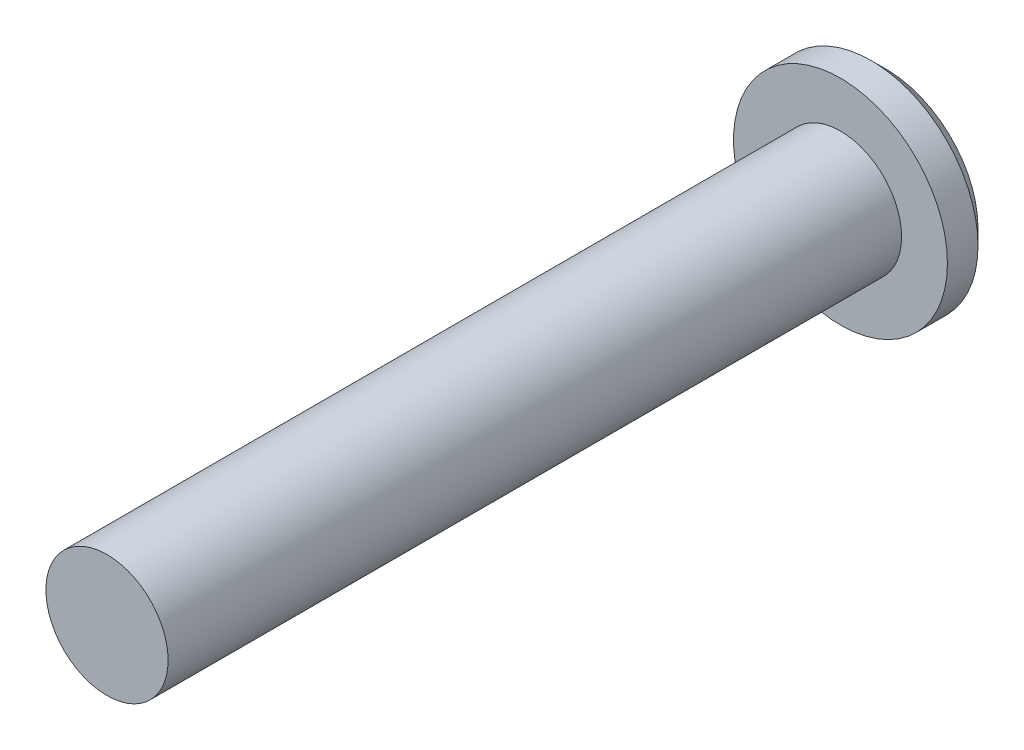
ISO-10303-21;
HEADER;
FILE_DESCRIPTION(('STEP AP214'),'2;1');
FILE_NAME('part.step','',(''),(''),'','','');
FILE_SCHEMA(('AUTOMOTIVE_DESIGN { 1 0 10303 214 1 1 1 1 }'));
ENDSEC;
DATA;
#1=APPLICATION_CONTEXT('core data for automotive mechanical design processes');
#2=APPLICATION_PROTOCOL_DEFINITION('international standard','automotive_design',2000,#1);
#3=PRODUCT_CONTEXT('',#1,'mechanical');
#4=PRODUCT('Part','Part','',(#3));
#5=PRODUCT_RELATED_PRODUCT_CATEGORY('part','',(#4));
#6=PRODUCT_DEFINITION_FORMATION('','',#4);
#7=PRODUCT_DEFINITION_CONTEXT('part definition',#1,'design');
#8=PRODUCT_DEFINITION('design','',#6,#7);
#9=PRODUCT_DEFINITION_SHAPE('','',#8);
#10=(LENGTH_UNIT() NAMED_UNIT(*) SI_UNIT(.MILLI.,.METRE.));
#11=(NAMED_UNIT(*) PLANE_ANGLE_UNIT() SI_UNIT($,.RADIAN.));
#12=(NAMED_UNIT(*) SI_UNIT($,.STERADIAN.) SOLID_ANGLE_UNIT());
#13=UNCERTAINTY_MEASURE_WITH_UNIT(LENGTH_MEASURE(1.E-05),#10,'distance_accuracy_value','');
#14=(GEOMETRIC_REPRESENTATION_CONTEXT(3) GLOBAL_UNCERTAINTY_ASSIGNED_CONTEXT((#13)) GLOBAL_UNIT_ASSIGNED_CONTEXT((#10,
#11,#12)) REPRESENTATION_CONTEXT('',''));
#15=CARTESIAN_POINT('',(0.,0.,0.));
#16=DIRECTION('',(0.,0.,1.));
#17=DIRECTION('',(1.,0.,0.));
#18=AXIS2_PLACEMENT_3D('',#15,#16,#17);
#19=CARTESIAN_POINT('',(0.,0.,3.));
#20=DIRECTION('',(0.,0.,-1.));
#21=DIRECTION('',(-1.,0.,0.));
#22=AXIS2_PLACEMENT_3D('',#19,#20,#21);
#23=CYLINDRICAL_SURFACE('',#22,7.);
#24=CARTESIAN_POINT('',(0.,0.,1.));
#25=DIRECTION('',(0.,0.,1.));
#26=DIRECTION('',(1.,0.,0.));
#27=AXIS2_PLACEMENT_3D('',#24,#25,#26);
#28=CIRCLE('',#27,7.);
#29=CARTESIAN_POINT('',(7.,0.,1.));
#30=VERTEX_POINT('',#29);
#31=EDGE_CURVE('E52',#30,#30,#28,.T.);
#32=ORIENTED_EDGE('',*,*,#31,.T.);
#33=EDGE_LOOP('',(#32));
#34=FACE_BOUND('',#33,.T.);
#35=CARTESIAN_POINT('',(0.,0.,3.));
#36=DIRECTION('',(0.,0.,1.));
#37=DIRECTION('',(1.,0.,0.));
#38=AXIS2_PLACEMENT_3D('',#35,#36,#37);
#39=CIRCLE('',#38,7.);
#40=CARTESIAN_POINT('',(7.,0.,3.));
#41=VERTEX_POINT('',#40);
#42=EDGE_CURVE('E61',#41,#41,#39,.T.);
#43=ORIENTED_EDGE('',*,*,#42,.F.);
#44=EDGE_LOOP('',(#43));
#45=FACE_BOUND('',#44,.T.);
#46=ADVANCED_FACE('F44',(#34,#45),#23,.T.);
#47=CARTESIAN_POINT('',(0.,0.,3.));
#48=DIRECTION('',(0.,0.,1.));
#49=DIRECTION('',(1.,0.,0.));
#50=AXIS2_PLACEMENT_3D('',#47,#48,#49);
#51=PLANE('',#50);
#52=CARTESIAN_POINT('',(0.,0.,3.));
#53=DIRECTION('',(0.,0.,1.));
#54=DIRECTION('',(1.,0.,0.));
#55=AXIS2_PLACEMENT_3D('',#52,#53,#54);
#56=CIRCLE('',#55,4.);
#57=CARTESIAN_POINT('',(4.,0.,3.));
#58=VERTEX_POINT('',#57);
#59=EDGE_CURVE('E60',#58,#58,#56,.T.);
#60=ORIENTED_EDGE('',*,*,#59,.F.);
#61=EDGE_LOOP('',(#60));
#62=FACE_BOUND('',#61,.T.);
#63=ORIENTED_EDGE('',*,*,#42,.T.);
#64=EDGE_LOOP('',(#63));
#65=FACE_BOUND('',#64,.T.);
#66=ADVANCED_FACE('F78',(#62,#65),#51,.T.);
#67=CARTESIAN_POINT('',(0.,0.,0.));
#68=DIRECTION('',(0.,0.,1.));
#69=DIRECTION('',(1.,0.,0.));
#70=AXIS2_PLACEMENT_3D('',#67,#68,#69);
#71=PLANE('',#70);
#72=CARTESIAN_POINT('',(0.,0.,0.));
#73=DIRECTION('',(0.,0.,1.));
#74=DIRECTION('',(1.,0.,0.));
#75=AXIS2_PLACEMENT_3D('',#72,#73,#74);
#76=CIRCLE('',#75,5.99999999999999);
#77=CARTESIAN_POINT('',(5.99999999999999,0.,0.));
#78=VERTEX_POINT('',#77);
#79=EDGE_CURVE('E10',#78,#78,#76,.F.);
#80=ORIENTED_EDGE('',*,*,#79,.T.);
#81=EDGE_LOOP('',(#80));
#82=FACE_BOUND('',#81,.T.);
#83=ADVANCED_FACE('F73',(#82),#71,.F.);
#84=CARTESIAN_POINT('',(0.,0.,51.));
#85=DIRECTION('',(0.,0.,-1.));
#86=DIRECTION('',(-1.,0.,0.));
#87=AXIS2_PLACEMENT_3D('',#84,#85,#86);
#88=CYLINDRICAL_SURFACE('',#87,4.);
#89=CARTESIAN_POINT('',(0.,0.,51.));
#90=DIRECTION('',(0.,0.,1.));
#91=DIRECTION('',(1.,0.,0.));
#92=AXIS2_PLACEMENT_3D('',#89,#90,#91);
#93=CIRCLE('',#92,4.);
#94=CARTESIAN_POINT('',(4.,0.,51.));
#95=VERTEX_POINT('',#94);
#96=EDGE_CURVE('E64',#95,#95,#93,.T.);
#97=ORIENTED_EDGE('',*,*,#96,.F.);
#98=EDGE_LOOP('',(#97));
#99=FACE_BOUND('',#98,.T.);
#100=ORIENTED_EDGE('',*,*,#59,.T.);
#101=EDGE_LOOP('',(#100));
#102=FACE_BOUND('',#101,.T.);
#103=ADVANCED_FACE('F75',(#99,#102),#88,.T.);
#104=CARTESIAN_POINT('',(0.,0.,51.));
#105=DIRECTION('',(0.,0.,1.));
#106=DIRECTION('',(1.,0.,0.));
#107=AXIS2_PLACEMENT_3D('',#104,#105,#106);
#108=PLANE('',#107);
#109=ORIENTED_EDGE('',*,*,#96,.T.);
#110=EDGE_LOOP('',(#109));
#111=FACE_BOUND('',#110,.T.);
#112=ADVANCED_FACE('F67',(#111),#108,.T.);
#113=CARTESIAN_POINT('',(0.,0.,1.));
#114=DIRECTION('',(0.,0.,1.));
#115=DIRECTION('',(1.,0.,0.));
#116=AXIS2_PLACEMENT_3D('',#113,#114,#115);
#117=CONICAL_SURFACE('',#116,7.,0.78539816339745);
#118=ORIENTED_EDGE('',*,*,#79,.F.);
#119=EDGE_LOOP('',(#118));
#120=FACE_BOUND('',#119,.T.);
#121=ORIENTED_EDGE('',*,*,#31,.F.);
#122=EDGE_LOOP('',(#121));
#123=FACE_BOUND('',#122,.T.);
#124=ADVANCED_FACE('F48',(#120,#123),#117,.T.);
#125=CLOSED_SHELL('',(#46,#66,#83,#103,#112,#124));
#126=MANIFOLD_SOLID_BREP('B2',#125);
#127=ADVANCED_BREP_SHAPE_REPRESENTATION('',(#18,#126),#14);
#128=SHAPE_DEFINITION_REPRESENTATION(#9,#127);
ENDSEC;
END-ISO-10303-21;
